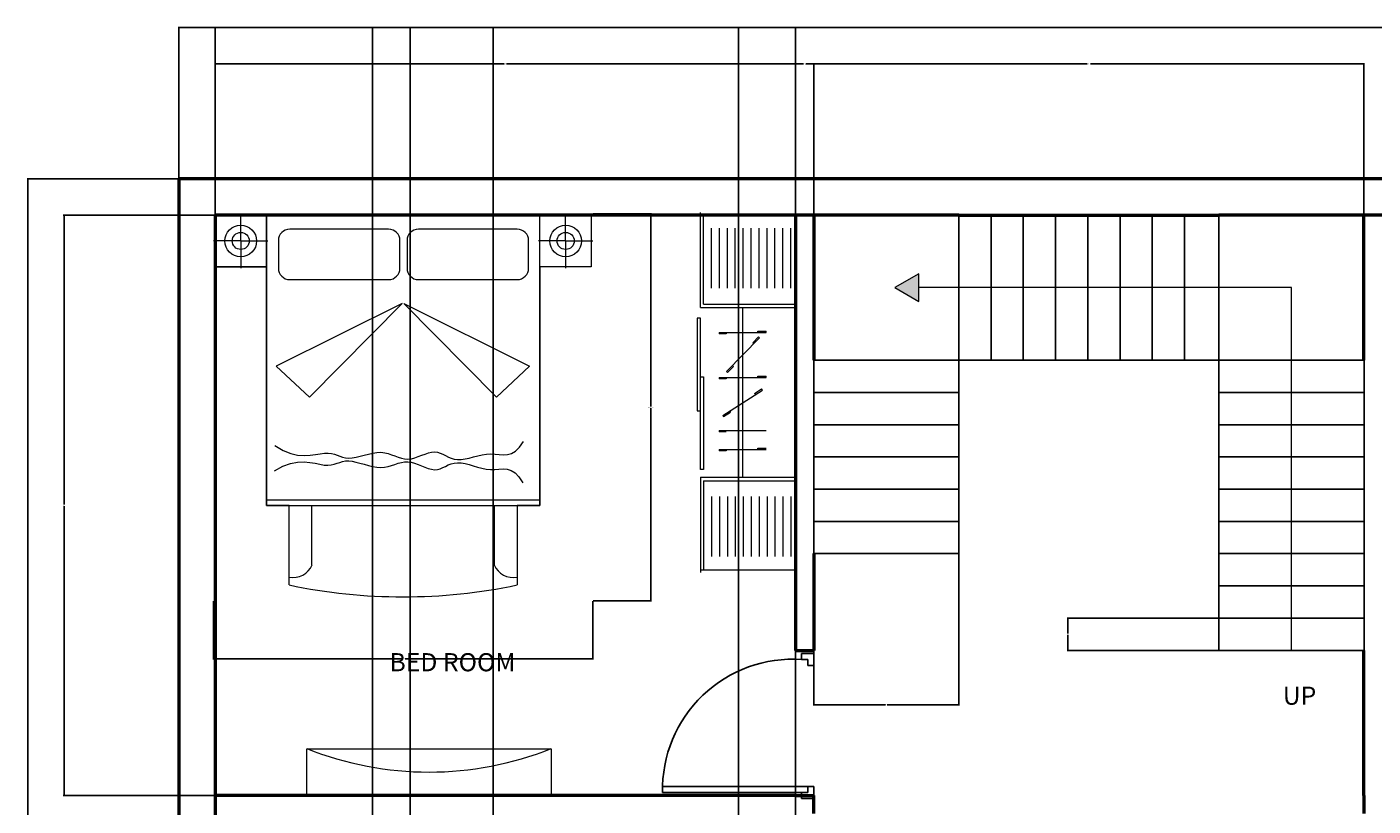
# Model space of a CAD drawing. Units: inches. Extents: x 1865 to 2541, y 1997 to 2759.
# Tile 8 of 11: x 1866 to 2200, y 2566 to 2759. Entities that reach past the tile are written whole.
import ezdxf

# ---------------------------------------------------------------- set-up
doc = ezdxf.new("R2010")
doc.units = ezdxf.units.IN
for name, color, linetype, lineweight in [('A-ANNO-DIMS', 2, 'Continuous', 18), ('A-ANNO-SYMB', 2, 'Continuous', 18), ('A-AREA-IDEN', 4, 'Continuous', 18), ('A-WALL', 7, 'Continuous', 50), ('BED', 42, 'Continuous', 13), ('CUPBOARD', 61, 'Continuous', 18), ('DOOR', 1, 'Continuous', 25), ('STAIRCASE', 2, 'Continuous', 25), ('TEXT', 4, 'Continuous', 18), ('TV', 3, 'Continuous', 18)]:
    doc.layers.add(name, color=color, linetype=linetype, lineweight=lineweight)
doc.styles.get("Standard").update_dxf_attribs({"font": 'arial.ttf'})
doc.dimstyles.get("Standard").update_dxf_attribs({"dimtxt": 0.18, "dimasz": 0.18, "dimexe": 0.18, "dimexo": 0.0625, "dimgap": 0.09, "dimtad": 0, "dimtih": 1, "dimtoh": 1, "dimdec": 4, "dimzin": 0, "dimdsep": 46, "dimtxsty": 'Standard', "dimcen": 0.09, "dimadec": 0, "dimazin": 0, "dimtfac": 1, "dimtdec": 4, "dimtofl": 0, "dimtmove": 0, "dimatfit": 3, "dimfxl": 1, "dimtolj": 1, "dimtzin": 0, "dimarcsym": 0})

# ---------------------------------------------------------------- blocks, each defined once
blk = doc.blocks.new('A$C4F543DC7')
for p, q in [((0.013, 3.35, -0.169), (3.313, 3.35, -0.169)), ((0.463, 3.35, -0.169), (0.013, 3.35, -0.169)), ((0.013, 2.896, -0.169), (0.013, 3.35, -0.169)), ((0.013, 3.35, -0.169), (0.013, 2.896, -0.169)), ((0.238, 3.123, -0.439), (0.238, 3.361, -0.439)), ((0.463, 3.35, -0.169), (0.463, 0.8, -0.169)), ((2.863, 3.35, -0.169), (0.463, 3.35, -0.169)), ((0.463, 2.896, -0.169), (0.463, 3.35, -0.169)), ((2.863, 0.8, -0.169), (2.863, 3.35, -0.169)), ((2.863, 3.35, -0.169), (3.313, 3.35, -0.169)), ((2.863, 2.896, -0.169), (2.863, 3.35, -0.169)), ((3.089, 3.123, -0.439), (3.089, 3.361, -0.439)), ((3.313, 3.35, -0.169), (3.313, 2.896, -0.169)), ((3.313, 3.35, -0.169), (3.313, 2.896, -0.169)), ((1.535, 3.226, -0.169), (0.668, 3.226, -0.169)), ((2.664, 3.226, -0.169), (1.797, 3.226, -0.169)), ((0.238, 3.123, -0.439), (0, 3.123, -0.439)), ((0.238, 3.123, -0.439), (0.476, 3.123, -0.439)), ((0.238, 3.123, -0.439), (0.238, 2.885, -0.439)), ((0.568, 3.126, -0.169), (0.568, 2.884, -0.169)), ((1.635, 2.884, -0.169), (1.635, 3.126, -0.169)), ((1.697, 3.126, -0.169), (1.697, 2.884, -0.169)), ((2.764, 2.884, -0.169), (2.764, 3.126, -0.169)), ((3.089, 3.123, -0.439), (2.851, 3.123, -0.439)), ((3.089, 3.123, -0.439), (3.089, 2.885, -0.439)), ((3.089, 3.123, -0.439), (3.327, 3.123, -0.439)), ((0.463, 2.896, -0.169), (0.013, 2.896, -0.169)), ((0.013, 2.896, -0.169), (0.463, 2.896, -0.169)), ((0.463, 0.8, -0.169), (0.463, 2.896, -0.169)), ((2.863, 2.896, -0.169), (2.863, 0.8, -0.169)), ((3.313, 2.896, -0.169), (2.863, 2.896, -0.169)), ((3.313, 2.896, -0.169), (2.863, 2.896, -0.169)), ((0.668, 2.784, -0.169), (1.535, 2.784, -0.169)), ((1.797, 2.784, -0.169), (2.664, 2.784, -0.169)), ((1.653, 2.573, -0.169), (0.55, 2.025, -0.169)), ((0.841, 1.752, -0.169), (1.653, 2.573, -0.169)), ((2.481, 1.752, -0.169), (1.669, 2.573, -0.169)), ((1.669, 2.573, -0.169), (2.772, 2.025, -0.169)), ((0.55, 2.025, -0.169), (0.841, 1.752, -0.169)), ((2.772, 2.025, -0.169), (2.481, 1.752, -0.169)), ((0.537, 1.327, -0.169), (0.609, 1.284, -0.169)), ((2.648, 1.277, -0.169), (2.683, 1.312, -0.169)), ((2.683, 1.312, -0.169), (2.718, 1.364, -0.169)), ((0.609, 1.284, -0.169), (0.676, 1.257, -0.169)), ((0.674, 1.171, -0.169), (0.736, 1.183, -0.169)), ((0.676, 1.257, -0.169), (0.737, 1.243, -0.169)), ((0.736, 1.183, -0.169), (0.793, 1.185, -0.169)), ((0.737, 1.243, -0.169), (0.794, 1.239, -0.169)), ((0.793, 1.185, -0.169), (0.845, 1.18, -0.169)), ((0.794, 1.239, -0.169), (0.846, 1.242, -0.169)), ((0.846, 1.242, -0.169), (0.893, 1.249, -0.169)), ((0.893, 1.249, -0.169), (0.935, 1.256, -0.169)), ((0.935, 1.256, -0.169), (0.972, 1.261, -0.169)), ((0.972, 1.261, -0.169), (1.004, 1.262, -0.169)), ((1.004, 1.262, -0.169), (1.033, 1.258, -0.169)), ((1.033, 1.258, -0.169), (1.06, 1.251, -0.169)), ((1.06, 1.251, -0.169), (1.084, 1.242, -0.169)), ((1.084, 1.242, -0.169), (1.108, 1.234, -0.169)), ((1.107, 1.18, -0.169), (1.132, 1.187, -0.169)), ((1.108, 1.234, -0.169), (1.132, 1.226, -0.169)), ((1.132, 1.226, -0.169), (1.158, 1.22, -0.169)), ((1.132, 1.187, -0.169), (1.157, 1.192, -0.169)), ((1.157, 1.192, -0.169), (1.185, 1.193, -0.169)), ((1.158, 1.22, -0.169), (1.185, 1.218, -0.169)), ((1.185, 1.218, -0.169), (1.216, 1.22, -0.169)), ((1.185, 1.193, -0.169), (1.216, 1.19, -0.169)), ((1.216, 1.22, -0.169), (1.25, 1.226, -0.169)), ((1.216, 1.19, -0.169), (1.249, 1.183, -0.169)), ((1.249, 1.183, -0.169), (1.284, 1.173, -0.169)), ((1.25, 1.226, -0.169), (1.285, 1.235, -0.169)), ((1.285, 1.235, -0.169), (1.322, 1.244, -0.169)), ((1.322, 1.244, -0.169), (1.359, 1.253, -0.169)), ((1.359, 1.253, -0.169), (1.396, 1.261, -0.169)), ((1.396, 1.261, -0.169), (1.433, 1.266, -0.169)), ((1.433, 1.266, -0.169), (1.468, 1.268, -0.169)), ((1.468, 1.268, -0.169), (1.501, 1.264, -0.169)), ((1.501, 1.264, -0.169), (1.532, 1.257, -0.169)), ((1.532, 1.257, -0.169), (1.562, 1.247, -0.169)), ((1.562, 1.247, -0.169), (1.591, 1.237, -0.169)), ((1.591, 1.237, -0.169), (1.62, 1.226, -0.169)), ((1.62, 1.226, -0.169), (1.648, 1.217, -0.169)), ((1.648, 1.217, -0.169), (1.676, 1.211, -0.169)), ((1.648, 1.18, -0.169), (1.676, 1.185, -0.169)), ((1.676, 1.211, -0.169), (1.705, 1.209, -0.169)), ((1.676, 1.185, -0.169), (1.705, 1.186, -0.169)), ((1.705, 1.209, -0.169), (1.735, 1.212, -0.169)), ((1.705, 1.186, -0.169), (1.734, 1.182, -0.169)), ((1.734, 1.182, -0.169), (1.764, 1.173, -0.169)), ((1.735, 1.212, -0.169), (1.765, 1.22, -0.169)), ((1.765, 1.22, -0.169), (1.795, 1.23, -0.169)), ((1.795, 1.23, -0.169), (1.826, 1.242, -0.169)), ((1.826, 1.242, -0.169), (1.856, 1.253, -0.169)), ((1.856, 1.253, -0.169), (1.885, 1.263, -0.169)), ((1.885, 1.263, -0.169), (1.913, 1.27, -0.169)), ((1.913, 1.27, -0.169), (1.94, 1.272, -0.169)), ((1.94, 1.272, -0.169), (1.965, 1.269, -0.169)), ((1.965, 1.269, -0.169), (1.989, 1.262, -0.169)), ((1.989, 1.262, -0.169), (2.012, 1.251, -0.169)), ((2.012, 1.251, -0.169), (2.036, 1.239, -0.169)), ((2.036, 1.239, -0.169), (2.06, 1.227, -0.169)), ((2.06, 1.227, -0.169), (2.085, 1.216, -0.169)), ((2.085, 1.216, -0.169), (2.112, 1.208, -0.169)), ((2.112, 1.208, -0.169), (2.141, 1.204, -0.169)), ((2.141, 1.204, -0.169), (2.172, 1.205, -0.169)), ((2.172, 1.205, -0.169), (2.206, 1.21, -0.169)), ((2.206, 1.21, -0.169), (2.242, 1.218, -0.169)), ((2.242, 1.218, -0.169), (2.279, 1.228, -0.169)), ((2.279, 1.228, -0.169), (2.317, 1.238, -0.169)), ((2.317, 1.238, -0.169), (2.356, 1.246, -0.169)), ((2.356, 1.246, -0.169), (2.394, 1.253, -0.169)), ((2.394, 1.253, -0.169), (2.433, 1.255, -0.169)), ((2.433, 1.255, -0.169), (2.47, 1.253, -0.169)), ((2.47, 1.253, -0.169), (2.506, 1.249, -0.169)), ((2.506, 1.249, -0.169), (2.542, 1.246, -0.169)), ((2.542, 1.246, -0.169), (2.578, 1.248, -0.169)), ((2.578, 1.248, -0.169), (2.613, 1.257, -0.169)), ((2.613, 1.257, -0.169), (2.648, 1.277, -0.169)), ((0.533, 1.105, -0.169), (0.607, 1.146, -0.169)), ((0.607, 1.146, -0.169), (0.674, 1.171, -0.169)), ((0.845, 1.18, -0.169), (0.891, 1.172, -0.169)), ((0.891, 1.172, -0.169), (0.933, 1.163, -0.169)), ((0.933, 1.163, -0.169), (0.97, 1.156, -0.169)), ((0.97, 1.156, -0.169), (1.003, 1.155, -0.169)), ((1.003, 1.155, -0.169), (1.032, 1.158, -0.169)), ((1.032, 1.158, -0.169), (1.058, 1.164, -0.169)), ((1.058, 1.164, -0.169), (1.083, 1.172, -0.169)), ((1.083, 1.172, -0.169), (1.107, 1.18, -0.169)), ((1.284, 1.173, -0.169), (1.321, 1.163, -0.169)), ((1.321, 1.163, -0.169), (1.358, 1.152, -0.169)), ((1.358, 1.152, -0.169), (1.394, 1.143, -0.169)), ((1.394, 1.143, -0.169), (1.431, 1.137, -0.169)), ((1.431, 1.137, -0.169), (1.466, 1.135, -0.169)), ((1.466, 1.135, -0.169), (1.499, 1.137, -0.169)), ((1.499, 1.137, -0.169), (1.531, 1.143, -0.169)), ((1.531, 1.143, -0.169), (1.561, 1.152, -0.169)), ((1.561, 1.152, -0.169), (1.59, 1.162, -0.169)), ((1.59, 1.162, -0.169), (1.619, 1.172, -0.169)), ((1.619, 1.172, -0.169), (1.648, 1.18, -0.169)), ((1.764, 1.173, -0.169), (1.794, 1.162, -0.169)), ((1.794, 1.162, -0.169), (1.824, 1.149, -0.169)), ((1.824, 1.149, -0.169), (1.854, 1.137, -0.169)), ((1.854, 1.137, -0.169), (1.883, 1.126, -0.169)), ((1.883, 1.126, -0.169), (1.911, 1.119, -0.169)), ((1.911, 1.119, -0.169), (1.937, 1.115, -0.169)), ((1.937, 1.115, -0.169), (1.963, 1.118, -0.169)), ((1.963, 1.118, -0.169), (1.987, 1.124, -0.169)), ((1.987, 1.124, -0.169), (2.011, 1.134, -0.169)), ((2.011, 1.134, -0.169), (2.034, 1.145, -0.169)), ((2.034, 1.145, -0.169), (2.059, 1.157, -0.169)), ((2.059, 1.157, -0.169), (2.084, 1.167, -0.169)), ((2.084, 1.167, -0.169), (2.111, 1.174, -0.169)), ((2.111, 1.174, -0.169), (2.14, 1.177, -0.169)), ((2.14, 1.177, -0.169), (2.172, 1.175, -0.169)), ((2.172, 1.175, -0.169), (2.206, 1.169, -0.169)), ((2.206, 1.169, -0.169), (2.241, 1.16, -0.169)), ((2.241, 1.16, -0.169), (2.278, 1.149, -0.169)), ((2.278, 1.149, -0.169), (2.316, 1.138, -0.169)), ((2.316, 1.138, -0.169), (2.354, 1.128, -0.169)), ((2.354, 1.128, -0.169), (2.392, 1.121, -0.169)), ((2.392, 1.121, -0.169), (2.43, 1.117, -0.169)), ((2.43, 1.117, -0.169), (2.468, 1.118, -0.169)), ((2.468, 1.118, -0.169), (2.504, 1.121, -0.169)), ((2.504, 1.121, -0.169), (2.54, 1.123, -0.169)), ((2.54, 1.123, -0.169), (2.576, 1.12, -0.169)), ((2.576, 1.12, -0.169), (2.611, 1.109, -0.169)), ((2.611, 1.109, -0.169), (2.645, 1.088, -0.169)), ((2.645, 1.088, -0.169), (2.679, 1.052, -0.169)), ((2.679, 1.052, -0.169), (2.712, 0.999, -0.169)), ((0.463, 0.85, -0.169), (2.863, 0.85, -0.169)), ((0.463, 0.8, -0.169), (2.863, 0.8, -0.169)), ((0.663, 0.8, -0.169), (0.463, 0.8, -0.169)), ((0.663, 0.8, -0.169), (2.663, 0.8, -0.169)), ((0.663, 0.104, -0.169), (0.663, 0.8, -0.169)), ((0.663, 0.104, -0.169), (0.663, 0.8, -0.169)), ((0.863, 0.281, -0.169), (0.863, 0.8, -0.169)), ((2.463, 0.8, -0.169), (2.463, 0.281, -0.169)), ((2.863, 0.8, -0.169), (2.663, 0.8, -0.169)), ((2.663, 0.8, -0.169), (2.663, 0.104, -0.169)), ((2.663, 0.8, -0.169), (2.663, 0.104, -0.169))]:
    blk.add_line(p, q)
for centre, radius in [((0.238, 3.123, -0.439), 0.139), ((0.238, 3.123, -0.439), 0.075), ((3.089, 3.123, -0.439), 0.139), ((3.089, 3.123, -0.439), 0.075)]:
    blk.add_circle(centre, radius)
for centre, radius, start, end in [((0.668, 3.126, -0.169), 0.1, 90, 180), ((1.535, 3.126, -0.169), 0.1, 0, 90), ((1.797, 3.126, -0.169), 0.1, 90, 180), ((2.664, 3.126, -0.169), 0.1, 0, 90), ((0.668, 2.884, -0.169), 0.1, 180, 270), ((1.535, 2.884, -0.169), 0.1, 270, 0), ((1.797, 2.884, -0.169), 0.1, 180, 270), ((2.664, 2.884, -0.169), 0.1, 270, 0), ((0.699, 0.347, -0.169), 0.177, 258.2616, 338.032), ((2.627, 0.347, -0.169), 0.177, 201.968, 281.7384), ((1.663, 4.86, -0.169), 4.86, 258.1252, 281.8748), ((1.663, 4.86, -0.169), 4.86, 258.1252, 281.8748)]:
    blk.add_arc(centre, radius, start, end)
blk = doc.blocks.new('A$C34930FF8')
at = {"ltscale": 0.05}
for p, q in [((0, 2252.4), (0, 16.8)), ((600, 2252.4), (0, 2252.4)), ((185.4, 1513), (185.4, 1521.5)), ((227.1, 1479.2), (233.2, 1485.2)), ((237.7, 1513), (237.7, 1521.5)), ((263.6, 1441.7), (269.7, 1447.7)), ((436.7, 1513), (436.7, 1504.4)), ((482.5, 1513), (482.5, 1504.4)), ((398.2, 1303.6), (392.1, 1297.6)), ((185.4, 1229.1), (185.4, 1237.7)), ((237.7, 1229.1), (237.7, 1237.7)), ((434.8, 1266.1), (428.7, 1260.1)), ((436.7, 1228.2), (436.7, 1219.7)), ((482.5, 1228.2), (482.5, 1219.7)), ((209.5, 1150.1), (214.1, 1157.3)), ((253.5, 1121.8), (258.1, 1129)), ((415.3, 1017.6), (410.6, 1010.5)), ((459.3, 989.3), (454.7, 982.1)), ((482.5, 894.9), (482.5, 886.3)), ((237.7, 775.3), (237.7, 783.9)), ((436.7, 775.3), (436.7, 766.8)), ((482.5, 775.3), (482.5, 766.8)), ((600, 16.8), (0, 16.8))]:
    blk.add_line(p, q, dxfattribs=at)
for p, q in [((580, 1690.9), (580, 2252.4)), ((600, 1669.3), (600, 2269.3)), ((30, 1790.9), (30, 2169.3)), ((80, 1790.9), (80, 2169.3)), ((130, 1790.9), (130, 2169.3)), ((180, 1790.9), (180, 2169.3)), ((230, 1790.9), (230, 2169.3)), ((280, 1790.9), (280, 2169.3)), ((330, 1790.9), (330, 2169.3)), ((380, 1790.9), (380, 2169.3)), ((430, 1790.9), (430, 2169.3)), ((480, 1790.9), (480, 2169.3)), ((530, 1790.9), (530, 2169.3)), ((580, 1690.9), (0, 1690.9)), ((600, 1669.3), (0, 1669.3)), ((335.4, 1666.1), (335.4, 603.1)), ((600, 1603.3), (620, 1603.3)), ((600, 1018.7), (600, 1603.3)), ((620, 1603.3), (620, 1018.7)), ((237.7, 1521.5), (185.4, 1521.5)), ((482.5, 1513), (185.4, 1513)), ((434.8, 1266.1), (227.4, 1478.9)), ((269.7, 1447.7), (233.2, 1485.2)), ((436.7, 1504.4), (482.5, 1504.4)), ((428.7, 1260.1), (392.1, 1297.6)), ((237.7, 1237.7), (185.4, 1237.7)), ((482.5, 1228.2), (185.4, 1228.2)), ((436.7, 1219.7), (482.5, 1219.7)), ((600, 1233.4), (580, 1233.4)), ((580, 1233.4), (580, 648.7)), ((600, 648.7), (600, 1233.4)), ((459.3, 989.3), (209.5, 1150.1)), ((258.1, 1129), (214.1, 1157.3)), ((620, 1018.7), (600, 1018.7)), ((454.7, 982.1), (410.6, 1010.5)), ((482.5, 894.9), (185.4, 894.9)), ((436.7, 886.3), (482.5, 886.3)), ((237.7, 783.9), (185.4, 783.9)), ((482.5, 775.3), (185.4, 775.3)), ((436.7, 766.8), (482.5, 766.8)), ((600, 600), (0, 600)), ((580, 648.7), (600, 648.7)), ((600, 600), (600, 0)), ((580, 578.3), (0, 578.3)), ((580, 578.3), (580, 16.8)), ((30, 478.3), (30, 100)), ((80, 478.3), (80, 100)), ((130, 478.3), (130, 100)), ((180, 478.3), (180, 100)), ((230, 478.3), (230, 100)), ((280, 478.3), (280, 100)), ((330, 478.3), (330, 100)), ((380, 478.3), (380, 100)), ((430, 478.3), (430, 100)), ((480, 478.3), (480, 100)), ((530, 478.3), (530, 100))]:
    blk.add_line(p, q)
blk = doc.blocks.new('DOOR-SWING-36IN')
for p, q in [((36.01, 34.5), (0.01, 34.5)), ((34.51, 36), (37.51, 36)), ((34.51, 34.5), (34.51, 36)), ((36.01, 34.5), (34.51, 34.5)), ((36.01, 33), (36.01, 34.5)), ((37.51, 36), (37.51, 33)), ((36.01, 33), (0.01, 33)), ((37.51, 33), (36.01, 33)), ((36.01, 1.5), (34.51, 1.5)), ((34.51, 1.5), (34.51, 0)), ((34.51, 0), (37.51, 0)), ((37.51, 3), (36.01, 3)), ((36.01, 3), (36.01, 1.5)), ((37.51, 0), (37.51, 3))]:
    blk.add_line(p, q)
blk.add_arc((32.32, 33.75), 32.32, 178.6705, 273.8756)
blk = doc.blocks.new('TV-UNIT')
blk.add_lwpolyline([(0, 11.62), (60.65, 11.62), (60.65, 0), (0, 0)], close=True)
blk.add_arc((30.32, -76.26), 82.06, 68.3146, 111.6854)
blk = doc.blocks.new('*D24')
at = {"layer": 'A-ANNO-DIMS', "color": 0, "lineweight": -2, "transparency": 16777216}
for p, q in [((2005.98, 2712.77), (2020.5, 2712.77)), ((2020.32, 2712.59), (2020.32, 2664.95)), ((2020.32, 2616.94), (2020.32, 2664.58)), ((2005.98, 2616.76), (2020.5, 2616.76))]:
    blk.add_line(p, q, dxfattribs=at)
at = {"layer": 'A-ANNO-DIMS', "color": 0, "transparency": 16777216}
for points in [[(2020.29, 2712.59), (2020.35, 2712.59), (2020.32, 2712.77)], [(2020.29, 2616.94), (2020.35, 2616.94), (2020.32, 2616.76)]]:
    blk.add_solid(points, dxfattribs=at)
at = {"layer": 'Defpoints', "color": 0, "transparency": 16777216}
for p in [(2005.92, 2712.77), (2020.32, 2712.77), (2005.92, 2616.76)]:
    blk.add_point(p, dxfattribs=at)
at = {"layer": 'A-ANNO-DIMS', "color": 0, "transparency": 16777216, "insert": (2020.32, 2664.76), "char_height": 0.18, "attachment_point": 5}
blk.add_mtext('\\A1;BED UNIT 96 TYP.', dxfattribs=at)
blk = doc.blocks.new('*D25')
at = {"layer": 'A-ANNO-DIMS', "color": 0, "lineweight": -2, "transparency": 16777216}
for p, q in [((1911.86, 2616.7), (1911.86, 2602.18)), ((2005.92, 2616.7), (2005.92, 2602.18)), ((1912.04, 2602.36), (1958.36, 2602.36)), ((2005.74, 2602.36), (1959.42, 2602.36))]:
    blk.add_line(p, q, dxfattribs=at)
at = {"layer": 'A-ANNO-DIMS', "color": 0, "transparency": 16777216}
for points in [[(1912.04, 2602.39), (1912.04, 2602.33), (1911.86, 2602.36)], [(2005.74, 2602.39), (2005.74, 2602.33), (2005.92, 2602.36)]]:
    blk.add_solid(points, dxfattribs=at)
at = {"layer": 'Defpoints', "color": 0, "transparency": 16777216}
for p in [(1911.86, 2616.76), (2005.92, 2616.76), (2005.92, 2602.36)]:
    blk.add_point(p, dxfattribs=at)
at = {"layer": 'A-ANNO-DIMS', "color": 0, "transparency": 16777216, "insert": (1958.89, 2602.36), "char_height": 0.18, "attachment_point": 5}
blk.add_mtext('\\A1;94 TYP.', dxfattribs=at)
blk = doc.blocks.new('*D40')
at = {"layer": 'A-ANNO-DIMS', "color": 0, "lineweight": -2, "transparency": 16777216}
for p, q in [((1903.24, 2721.51), (1903.24, 2759.13)), ((1903.42, 2758.95), (2202.95, 2758.95)), ((2503.06, 2758.95), (2203.53, 2758.95)), ((2503.24, 2721.51), (2503.24, 2759.13))]:
    blk.add_line(p, q, dxfattribs=at)
at = {"layer": 'A-ANNO-DIMS', "color": 0, "transparency": 16777216}
for points in [[(1903.42, 2758.98), (1903.42, 2758.92), (1903.24, 2758.95)], [(2503.06, 2758.98), (2503.06, 2758.92), (2503.24, 2758.95)]]:
    blk.add_solid(points, dxfattribs=at)
at = {"layer": 'Defpoints', "color": 0, "transparency": 16777216}
for p in [(2503.24, 2758.95), (1903.24, 2721.45), (2503.24, 2721.45)]:
    blk.add_point(p, dxfattribs=at)
at = {"layer": 'A-ANNO-DIMS', "color": 0, "transparency": 16777216, "insert": (2203.24, 2758.95), "char_height": 0.18, "attachment_point": 5}
blk.add_mtext('\\A1;600', dxfattribs=at)
blk = doc.blocks.new('*D41')
at = {"layer": 'A-ANNO-DIMS', "color": 0, "lineweight": -2, "transparency": 16777216}
for p, q in [((2503.31, 2721.45), (2540.92, 2721.45)), ((2540.74, 2721.27), (2540.74, 2378.49)), ((2540.74, 2035.35), (2540.74, 2378.13)), ((2136.19, 2035.17), (2540.92, 2035.17))]:
    blk.add_line(p, q, dxfattribs=at)
at = {"layer": 'A-ANNO-DIMS', "color": 0, "transparency": 16777216}
for points in [[(2540.71, 2721.27), (2540.77, 2721.27), (2540.74, 2721.45)], [(2540.71, 2035.35), (2540.77, 2035.35), (2540.74, 2035.17)]]:
    blk.add_solid(points, dxfattribs=at)
at = {"layer": 'Defpoints', "color": 0, "transparency": 16777216}
for p in [(2503.24, 2721.45), (2136.13, 2035.17), (2540.74, 2035.17)]:
    blk.add_point(p, dxfattribs=at)
at = {"layer": 'A-ANNO-DIMS', "color": 0, "transparency": 16777216, "insert": (2540.74, 2378.31), "char_height": 0.18, "attachment_point": 5}
blk.add_mtext('\\A1;686.3', dxfattribs=at)
blk = doc.blocks.new('*D42')
at = {"layer": 'A-ANNO-DIMS', "color": 0, "lineweight": -2, "transparency": 16777216}
for p, q in [((1903.18, 2721.45), (1865.56, 2721.45)), ((1865.74, 2721.27), (1865.74, 2391.63)), ((1865.74, 2061.63), (1865.74, 2391.27)), ((1903.18, 2061.45), (1865.56, 2061.45))]:
    blk.add_line(p, q, dxfattribs=at)
at = {"layer": 'A-ANNO-DIMS', "color": 0, "transparency": 16777216}
for points in [[(1865.71, 2721.27), (1865.77, 2721.27), (1865.74, 2721.45)], [(1865.71, 2061.63), (1865.77, 2061.63), (1865.74, 2061.45)]]:
    blk.add_solid(points, dxfattribs=at)
at = {"layer": 'Defpoints', "color": 0, "transparency": 16777216}
for p in [(1865.74, 2721.45), (1903.24, 2721.45), (1903.24, 2061.45)]:
    blk.add_point(p, dxfattribs=at)
at = {"layer": 'A-ANNO-DIMS', "color": 0, "transparency": 16777216, "insert": (1865.74, 2391.45), "char_height": 0.18, "attachment_point": 5}
blk.add_mtext('\\A1;660', dxfattribs=at)
blk = doc.blocks.new('*D43')
at = {"layer": 'A-ANNO-DIMS', "color": 0, "lineweight": -2, "transparency": 16777216}
for p, q in [((1912.24, 2712.51), (1912.24, 2750.13)), ((1912.42, 2749.95), (1983.96, 2749.95)), ((2056.06, 2749.95), (1984.52, 2749.95)), ((2056.24, 2712.51), (2056.24, 2750.13))]:
    blk.add_line(p, q, dxfattribs=at)
at = {"layer": 'A-ANNO-DIMS', "color": 0, "transparency": 16777216}
for points in [[(1912.42, 2749.98), (1912.42, 2749.92), (1912.24, 2749.95)], [(2056.06, 2749.98), (2056.06, 2749.92), (2056.24, 2749.95)]]:
    blk.add_solid(points, dxfattribs=at)
at = {"layer": 'Defpoints', "color": 0, "transparency": 16777216}
for p in [(2056.24, 2749.95), (1912.24, 2712.45), (2056.24, 2712.45)]:
    blk.add_point(p, dxfattribs=at)
at = {"layer": 'A-ANNO-DIMS', "color": 0, "transparency": 16777216, "insert": (1984.24, 2749.95), "char_height": 0.18, "attachment_point": 5}
blk.add_mtext('\\A1;144', dxfattribs=at)
blk = doc.blocks.new('*D44')
at = {"layer": 'A-ANNO-DIMS', "color": 0, "lineweight": -2, "transparency": 16777216}
for p, q in [((2060.74, 2712.51), (2060.74, 2750.13)), ((2060.92, 2749.95), (2128.61, 2749.95)), ((2197.06, 2749.95), (2129.38, 2749.95)), ((2197.24, 2712.51), (2197.24, 2750.13))]:
    blk.add_line(p, q, dxfattribs=at)
at = {"layer": 'A-ANNO-DIMS', "color": 0, "transparency": 16777216}
for points in [[(2060.92, 2749.98), (2060.92, 2749.92), (2060.74, 2749.95)], [(2197.06, 2749.98), (2197.06, 2749.92), (2197.24, 2749.95)]]:
    blk.add_solid(points, dxfattribs=at)
at = {"layer": 'Defpoints', "color": 0, "transparency": 16777216}
for p in [(2197.24, 2749.95), (2060.74, 2712.45), (2197.24, 2712.45)]:
    blk.add_point(p, dxfattribs=at)
at = {"layer": 'A-ANNO-DIMS', "color": 0, "transparency": 16777216, "insert": (2128.99, 2749.95), "char_height": 0.18, "attachment_point": 5}
blk.add_mtext('\\A1;136.5', dxfattribs=at)
blk = doc.blocks.new('*D47')
at = {"layer": 'A-ANNO-DIMS', "color": 0, "lineweight": -2, "transparency": 16777216}
for p, q in [((1912.18, 2712.45), (1874.56, 2712.45)), ((1874.74, 2712.27), (1874.74, 2640.63)), ((1874.74, 2568.63), (1874.74, 2640.27)), ((1912.18, 2568.45), (1874.56, 2568.45))]:
    blk.add_line(p, q, dxfattribs=at)
at = {"layer": 'A-ANNO-DIMS', "color": 0, "transparency": 16777216}
for points in [[(1874.71, 2712.27), (1874.77, 2712.27), (1874.74, 2712.45)], [(1874.71, 2568.63), (1874.77, 2568.63), (1874.74, 2568.45)]]:
    blk.add_solid(points, dxfattribs=at)
at = {"layer": 'Defpoints', "color": 0, "transparency": 16777216}
for p in [(1874.74, 2712.45), (1912.24, 2712.45), (1912.24, 2568.45)]:
    blk.add_point(p, dxfattribs=at)
at = {"layer": 'A-ANNO-DIMS', "color": 0, "transparency": 16777216, "insert": (1874.74, 2640.45), "char_height": 0.18, "attachment_point": 5}
blk.add_mtext('\\A1;144', dxfattribs=at)
blk = doc.blocks.new('*D60')
at = {"layer": 'A-ANNO-DIMS', "color": 0, "lineweight": -2, "transparency": 16777216}
for p, q in [((2056.24, 2712.51), (2056.24, 2750.13)), ((2056.42, 2749.95), (2058.23, 2749.95)), ((2060.56, 2749.95), (2058.75, 2749.95)), ((2060.74, 2712.51), (2060.74, 2750.13))]:
    blk.add_line(p, q, dxfattribs=at)
at = {"layer": 'A-ANNO-DIMS', "color": 0, "transparency": 16777216}
for points in [[(2056.42, 2749.98), (2056.42, 2749.92), (2056.24, 2749.95)], [(2060.56, 2749.98), (2060.56, 2749.92), (2060.74, 2749.95)]]:
    blk.add_solid(points, dxfattribs=at)
at = {"layer": 'Defpoints', "color": 0, "transparency": 16777216}
for p in [(2060.74, 2749.95), (2056.24, 2712.45), (2060.74, 2712.45)]:
    blk.add_point(p, dxfattribs=at)
at = {"layer": 'A-ANNO-DIMS', "color": 0, "transparency": 16777216, "insert": (2058.49, 2749.95), "char_height": 0.18, "attachment_point": 5}
blk.add_mtext('\\A1;4.5', dxfattribs=at)
blk = doc.blocks.new('*D68')
at = {"layer": 'A-ANNO-DIMS', "color": 0, "lineweight": -2, "transparency": 16777216}
for p, q in [((1912.24, 2169.51), (1912.24, 2759.13)), ((1912.42, 2758.95), (1931.52, 2758.95)), ((1951.06, 2758.95), (1931.96, 2758.95)), ((1951.24, 2169.51), (1951.24, 2759.13))]:
    blk.add_line(p, q, dxfattribs=at)
at = {"layer": 'A-ANNO-DIMS', "color": 0, "transparency": 16777216}
for points in [[(1912.42, 2758.98), (1912.42, 2758.92), (1912.24, 2758.95)], [(1951.06, 2758.98), (1951.06, 2758.92), (1951.24, 2758.95)]]:
    blk.add_solid(points, dxfattribs=at)
at = {"layer": 'Defpoints', "color": 0, "transparency": 16777216}
for p in [(1951.24, 2758.95), (1912.24, 2169.45), (1951.24, 2169.45)]:
    blk.add_point(p, dxfattribs=at)
at = {"layer": 'A-ANNO-DIMS', "color": 0, "transparency": 16777216, "insert": (1931.74, 2758.95), "char_height": 0.18, "attachment_point": 5}
blk.add_mtext('\\A1;39', dxfattribs=at)
blk = doc.blocks.new('*D69')
at = {"layer": 'A-ANNO-DIMS', "color": 0, "lineweight": -2, "transparency": 16777216}
for p, q in [((2060.74, 2628.39), (2060.74, 2590.77)), ((2096.74, 2628.39), (2096.74, 2590.77)), ((2060.92, 2590.95), (2078.52, 2590.95)), ((2096.56, 2590.95), (2078.96, 2590.95))]:
    blk.add_line(p, q, dxfattribs=at)
at = {"layer": 'A-ANNO-DIMS', "color": 0, "transparency": 16777216}
for points in [[(2060.92, 2590.98), (2060.92, 2590.92), (2060.74, 2590.95)], [(2096.56, 2590.98), (2096.56, 2590.92), (2096.74, 2590.95)]]:
    blk.add_solid(points, dxfattribs=at)
at = {"layer": 'Defpoints', "color": 0, "transparency": 16777216}
for p in [(2060.74, 2628.45), (2096.74, 2628.45), (2060.74, 2590.95)]:
    blk.add_point(p, dxfattribs=at)
at = {"layer": 'A-ANNO-DIMS', "color": 0, "transparency": 16777216, "insert": (2078.74, 2590.95), "char_height": 0.18, "attachment_point": 5}
blk.add_mtext('\\A1;36', dxfattribs=at)
blk = doc.blocks.new('*D70')
at = {"layer": 'A-ANNO-DIMS', "color": 0, "lineweight": -2, "transparency": 16777216}
for p, q in [((2161.22, 2612.45), (2123.6, 2612.45)), ((2123.78, 2612.27), (2123.78, 2608.63)), ((2123.78, 2604.63), (2123.78, 2608.27)), ((2161.22, 2604.45), (2123.6, 2604.45))]:
    blk.add_line(p, q, dxfattribs=at)
at = {"layer": 'A-ANNO-DIMS', "color": 0, "transparency": 16777216}
for points in [[(2123.75, 2612.27), (2123.81, 2612.27), (2123.78, 2612.45)], [(2123.75, 2604.63), (2123.81, 2604.63), (2123.78, 2604.45)]]:
    blk.add_solid(points, dxfattribs=at)
at = {"layer": 'Defpoints', "color": 0, "transparency": 16777216}
for p in [(2123.78, 2612.45), (2161.28, 2612.45), (2161.28, 2604.45)]:
    blk.add_point(p, dxfattribs=at)
at = {"layer": 'A-ANNO-DIMS', "color": 0, "transparency": 16777216, "insert": (2123.78, 2608.45), "char_height": 0.18, "attachment_point": 5}
blk.add_mtext('\\A1;8', dxfattribs=at)
blk = doc.blocks.new('*D81')
at = {"layer": 'A-ANNO-DIMS', "color": 0, "lineweight": -2, "transparency": 16777216}
for p, q in [((1960.58, 2070.51), (1960.58, 2759.13)), ((1960.76, 2758.95), (1970.44, 2758.95)), ((1981.06, 2758.95), (1971.38, 2758.95)), ((1981.24, 2070.51), (1981.24, 2759.13))]:
    blk.add_line(p, q, dxfattribs=at)
at = {"layer": 'A-ANNO-DIMS', "color": 0, "transparency": 16777216}
for points in [[(1960.76, 2758.98), (1960.76, 2758.92), (1960.58, 2758.95)], [(1981.06, 2758.98), (1981.06, 2758.92), (1981.24, 2758.95)]]:
    blk.add_solid(points, dxfattribs=at)
at = {"layer": 'Defpoints', "color": 0, "transparency": 16777216}
for p in [(1960.58, 2758.95), (1960.58, 2070.45), (1981.24, 2070.45)]:
    blk.add_point(p, dxfattribs=at)
at = {"layer": 'A-ANNO-DIMS', "color": 0, "transparency": 16777216, "insert": (1970.91, 2758.95), "char_height": 0.18, "attachment_point": 5}
blk.add_mtext('\\A1;20.665', dxfattribs=at)
blk = doc.blocks.new('*D82')
at = {"layer": 'A-ANNO-DIMS', "color": 0, "lineweight": -2, "transparency": 16777216}
for p, q in [((2042.07, 2070.51), (2042.07, 2759.13)), ((2042.25, 2758.95), (2048.7, 2758.95)), ((2056.06, 2758.95), (2049.61, 2758.95)), ((2056.24, 2070.51), (2056.24, 2759.13))]:
    blk.add_line(p, q, dxfattribs=at)
at = {"layer": 'A-ANNO-DIMS', "color": 0, "transparency": 16777216}
for points in [[(2042.25, 2758.98), (2042.25, 2758.92), (2042.07, 2758.95)], [(2056.06, 2758.98), (2056.06, 2758.92), (2056.24, 2758.95)]]:
    blk.add_solid(points, dxfattribs=at)
at = {"layer": 'Defpoints', "color": 0, "transparency": 16777216}
for p in [(2042.07, 2758.95), (2042.07, 2070.45), (2056.24, 2070.45)]:
    blk.add_point(p, dxfattribs=at)
at = {"layer": 'A-ANNO-DIMS', "color": 0, "transparency": 16777216, "insert": (2049.16, 2758.95), "char_height": 0.18, "attachment_point": 5}
blk.add_mtext('\\A1;14.176', dxfattribs=at)

msp = doc.modelspace()

# ---------------------------------------------------------------- hatches: boundary and pattern name
at = {"layer": 'A-ANNO-SYMB'}
h = msp.add_hatch(color=256, dxfattribs=at)
h.dxf.hatch_style = 1
h.paths.add_polyline_path([(2086.8433, 2690.9883), (2086.8433, 2697.9105), (2080.8485, 2694.4494)])

# ---------------------------------------------------------------- linework, layer by layer
for p, q in [((2179.2838, 2694.4494), (2086.8433, 2694.4494)), ((2179.2838, 2604.4494), (2179.2838, 2694.4494))]:
    msp.add_line(p, q, dxfattribs=at)
msp.add_lwpolyline([(2086.8433, 2690.9883), (2086.8433, 2697.9105), (2080.8485, 2694.4494)], close=True, dxfattribs=at)
at = {"layer": 'A-WALL'}
for p, q in [((2503.243, 2721.4494), (1903.243, 2721.4494)), ((1903.243, 2721.4494), (1903.243, 2061.4494)), ((1912.243, 2712.4494), (1912.243, 2406.9494)), ((2096.743, 2712.4494), (1912.243, 2712.4494)), ((2056.243, 2712.4494), (2056.243, 2604.4494)), ((2060.743, 2712.4494), (2060.743, 2676.4494)), ((2096.743, 2712.4494), (2161.2838, 2712.4494)), ((2494.243, 2712.4494), (2161.2838, 2712.4494)), ((2197.243, 2676.4494), (2197.243, 2712.4494)), ((2060.743, 2628.4494), (2060.743, 2604.4494)), ((2056.243, 2604.4494), (2060.743, 2604.4494)), ((2197.243, 2568.4494), (2197.243, 2604.4494)), ((2056.243, 2568.4494), (1912.243, 2568.4494)), ((2056.243, 2568.4494), (2060.743, 2568.4494)), ((2060.743, 2563.9494), (2060.743, 2568.4494)), ((2197.243, 2568.4494), (2197.243, 2563.9494))]:
    msp.add_line(p, q, dxfattribs=at)
at = {"layer": 'STAIRCASE'}
for p, q in [((2096.743, 2712.4494), (2060.743, 2712.4494)), ((2060.743, 2712.4494), (2060.743, 2676.4494)), ((2096.743, 2676.4494), (2096.743, 2712.4494)), ((2104.743, 2676.4494), (2104.743, 2712.4494)), ((2112.743, 2676.4494), (2112.743, 2712.4494)), ((2120.743, 2676.4494), (2120.743, 2712.4494)), ((2128.743, 2676.4494), (2128.743, 2712.4494)), ((2136.743, 2676.4494), (2136.743, 2712.4494)), ((2144.743, 2676.4494), (2144.743, 2712.4494)), ((2152.743, 2676.4494), (2152.743, 2712.4494)), ((2197.2838, 2712.4494), (2161.2838, 2712.4494)), ((2161.2838, 2712.4494), (2161.2838, 2676.4494)), ((2197.2838, 2676.4494), (2197.2838, 2712.4494)), ((2060.743, 2676.4494), (2096.743, 2676.4494)), ((2060.743, 2676.4494), (2060.743, 2628.4494)), ((2096.743, 2676.4494), (2096.743, 2628.4494)), ((2096.743, 2676.4494), (2161.2838, 2676.4494)), ((2161.2838, 2676.4494), (2197.2838, 2676.4494)), ((2161.2838, 2676.4494), (2161.2838, 2604.4494)), ((2197.2838, 2676.4494), (2197.2838, 2604.4494)), ((2060.743, 2668.4494), (2096.743, 2668.4494)), ((2161.2838, 2668.4494), (2197.2838, 2668.4494)), ((2060.743, 2660.4494), (2096.743, 2660.4494)), ((2161.2838, 2660.4494), (2197.2838, 2660.4494)), ((2060.743, 2652.4494), (2096.743, 2652.4494)), ((2161.2838, 2652.4494), (2197.2838, 2652.4494)), ((2060.743, 2644.4494), (2096.743, 2644.4494)), ((2161.2838, 2644.4494), (2197.2838, 2644.4494)), ((2060.743, 2636.4494), (2096.743, 2636.4494)), ((2161.2838, 2636.4494), (2197.2838, 2636.4494)), ((2060.743, 2628.4494), (2096.743, 2628.4494)), ((2161.2838, 2628.4494), (2197.2838, 2628.4494)), ((2161.2838, 2620.4494), (2197.2838, 2620.4494)), ((2161.2838, 2612.4494), (2197.2838, 2612.4494)), ((2161.2838, 2604.4494), (2197.2838, 2604.4494))]:
    msp.add_line(p, q, dxfattribs=at)

# ---------------------------------------------------------------- block references
at = {"layer": 'BED', "xscale": 28.27205529407425, "yscale": 28.27205529407425, "zscale": 28.27205529407425}
msp.add_blockref('A$C4F543DC7', (1911.8631, 2617.738, 4.7709), dxfattribs=at)
at = {"layer": 'CUPBOARD', "xscale": -0.0393700787401575, "yscale": 0.0393700787401575, "zscale": 0.0393700787401575}
msp.add_blockref('A$C34930FF8', (2056.243, 2623.7716), dxfattribs=at)
at = {"layer": 'DOOR', "extrusion": (0, 0, -1), "zscale": -1, "rotation": 180}
msp.add_blockref('DOOR-SWING-36IN', (-2023.234, 2603.6999), dxfattribs=at)
at = {"layer": 'TV', "rotation": 180}
msp.add_blockref('TV-UNIT', (1995.6253, 2580.0649), dxfattribs=at)

# ---------------------------------------------------------------- texts
at = {"layer": 'A-AREA-IDEN', "insert": (1955.5004, 2603.7636), "char_height": 4.5, "attachment_point": 1}
msp.add_mtext_dynamic_manual_height_columns('BED ROOM', width=66.075761, gutter_width=12.5, heights=[0], dxfattribs=at)
at = {"layer": 'TEXT', "insert": (2177.1145, 2595.4546), "char_height": 4.5, "attachment_point": 1}
msp.add_mtext_dynamic_manual_height_columns('UP', width=66.075761, gutter_width=12.5, heights=[0], dxfattribs=at)

# ---------------------------------------------------------------- dimensions: what is measured, and where the dimension line sits
at = {"layer": 'A-ANNO-DIMS'}
for base, p1, p2, override, picture, middle in [((2503.243, 2758.9494), (1903.243, 2721.4494), (2503.243, 2721.4494), {"dimdec": 0, "dimlfac": 1, "dimrnd": 0, "dimzin": 0, "dimdsep": 46, "dimlunit": 2}, '*D40', (2203.243, 2758.9494)), ((1951.243, 2758.9494), (1912.243, 2169.4494), (1951.243, 2169.4494), {"dimdec": 0, "dimlfac": 1, "dimrnd": 0, "dimzin": 0, "dimdsep": 46, "dimlunit": 2}, '*D68', (1931.743, 2758.9494)), ((1960.57848, 2758.94943), (1981.243, 2070.44943), (1960.57848, 2070.44943), {"dimdec": 3, "dimlfac": 1, "dimrnd": 0, "dimzin": 0, "dimdsep": 46, "dimlunit": 2}, '*D81', (1970.91074, 2758.94943)), ((2042.0671, 2758.9494), (2056.243, 2070.4494), (2042.0671, 2070.4494), {"dimdec": 3, "dimlfac": 1, "dimrnd": 0, "dimzin": 0, "dimdsep": 46, "dimlunit": 2}, '*D82', (2049.1551, 2758.9494)), ((2056.243, 2749.9494), (1912.243, 2712.4494), (2056.243, 2712.4494), {"dimdec": 0, "dimlfac": 1, "dimrnd": 0, "dimzin": 0, "dimdsep": 46, "dimlunit": 2}, '*D43', (1984.243, 2749.9494)), ((2060.743, 2749.9494), (2056.243, 2712.4494), (2060.743, 2712.4494), {"dimdec": 1, "dimlfac": 1, "dimrnd": 0, "dimzin": 0, "dimdsep": 46, "dimlunit": 2}, '*D60', (2058.493, 2749.9494)), ((2197.243, 2749.9494), (2060.743, 2712.4494), (2197.243, 2712.4494), {"dimdec": 1, "dimlfac": 1, "dimrnd": 0, "dimzin": 0, "dimdsep": 46, "dimlunit": 2}, '*D44', (2128.993, 2749.9494))]:
    dim = msp.add_linear_dim(base=base, p1=p1, p2=p2, dimstyle='Standard', override=override, dxfattribs=at)
    dim.commit()
    dim.dimension.update_dxf_attribs({"geometry": picture, "text_midpoint": middle})
for base, p1, p2, angle, override, picture, middle in [((1865.743, 2721.4494), (1903.243, 2061.4494), (1903.243, 2721.4494), 90, {"dimdec": 0, "dimlfac": 1, "dimrnd": 0, "dimzin": 0, "dimdsep": 46, "dimlunit": 2}, '*D42', (1865.743, 2391.4494)), ((2540.743, 2035.1708), (2503.243, 2721.4494), (2136.13, 2035.1708), 90, {"dimdec": 1, "dimlfac": 1, "dimrnd": 0, "dimzin": 0, "dimdsep": 46, "dimlunit": 2}, '*D41', (2540.743, 2378.3101)), ((1874.743, 2712.4494), (1912.243, 2568.4494), (1912.243, 2712.4494), 90, {"dimdec": 0, "dimlfac": 1, "dimrnd": 0, "dimzin": 0, "dimdsep": 46, "dimlunit": 2}, '*D47', (1874.743, 2640.4494)), ((2060.743, 2590.9494), (2096.743, 2628.4494), (2060.743, 2628.4494), 180, {"dimdec": 0, "dimlfac": 1, "dimrnd": 0, "dimzin": 0, "dimdsep": 46, "dimlunit": 2}, '*D69', (2078.743, 2590.9494)), ((2123.7838, 2612.4494), (2161.2838, 2604.4494), (2161.2838, 2612.4494), 90, {"dimdec": 0, "dimlfac": 1, "dimrnd": 0, "dimzin": 0, "dimdsep": 46, "dimlunit": 2}, '*D70', (2123.7838, 2608.4494))]:
    dim = msp.add_linear_dim(base=base, p1=p1, p2=p2, angle=angle, dimstyle='Standard', override=override, dxfattribs=at)
    dim.commit()
    dim.dimension.update_dxf_attribs({"geometry": picture, "text_midpoint": middle})
dim = msp.add_linear_dim(base=(2020.3227, 2712.7711), p1=(2005.9207, 2616.7579), p2=(2005.9207, 2712.7711), angle=90, text='BED UNIT <> TYP.', dimstyle='Standard', override={"dimdec": 0, "dimlfac": 1, "dimrnd": 0, "dimzin": 0, "dimdsep": 46, "dimlunit": 2}, dxfattribs=at)
dim.commit()
dim.dimension.update_dxf_attribs({"geometry": '*D24', "text_midpoint": (2020.3227, 2664.7645)})
dim = msp.add_linear_dim(base=(2005.9207, 2602.356), p1=(1911.8631, 2616.7579), p2=(2005.9207, 2616.7579), text='<> TYP.', dimstyle='Standard', override={"dimdec": 0, "dimlfac": 1, "dimrnd": 0, "dimzin": 0, "dimdsep": 46, "dimlunit": 2}, dxfattribs=at)
dim.commit()
dim.dimension.update_dxf_attribs({"geometry": '*D25', "text_midpoint": (1958.8919, 2602.356)})

doc.saveas('drawing.dxf')
